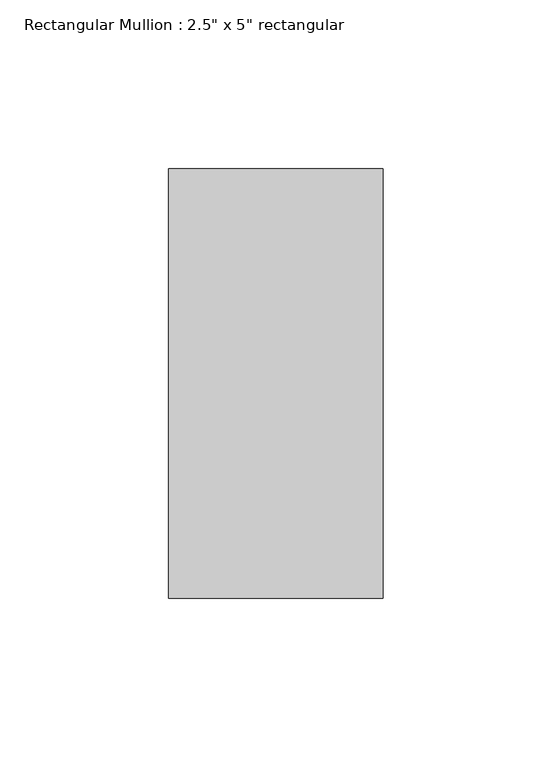
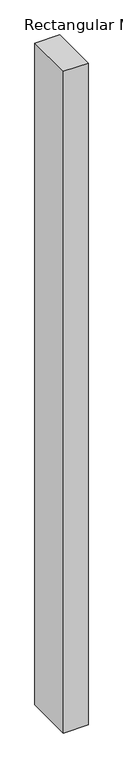
"""IFC4 building model written with IfcOpenShell, lengths in millimetres: member geometry."""

from ifc_helpers import new_model, si_unit, frame, origin, place, context, project, spatial, polyline, outline, extrude, source, transform, mapped, element, save


def member_5095b95d(model_context):
    return source(origin(), model_context, "Body", "SweptSolid", [
        extrude(outline(polyline([(31.75, 63.5), (31.75, -63.5), (-31.75, -63.5), (-31.75, 63.5), (31.75, 63.5)])), frame((0.0, 0.0, -1801.1599467), z_axis=(0.0, 0.0, 1.0), x_axis=(1.0, 0.0, 0.0)), (0.0, 0.0, 1.0), 1801.1599467),
    ])


if __name__ == "__main__":
    model = new_model("IFC4")
    model_context = context("Model", 3, world=origin())
    ifc_project = project(units=[si_unit("LENGTHUNIT", "METRE", prefix="MILLI")], contexts=[model_context])
    site = spatial("IfcSite", under=ifc_project)
    building = spatial("IfcBuilding", under=site)
    placement = place(None, origin())
    member_shape = member_5095b95d(model_context)
    element("IfcMember", 1, ObjectType="Rectangular Mullion : 2.5\" x 5\" rectangular", at=placement, inside=building, context=model_context, shape_type="MappedRepresentation", body=[
        mapped(member_shape, transform((0.0, 0.0, 0.0), x_axis=(1.0, 0.0, 0.0), y_axis=(0.0, 1.0, 0.0), z_axis=(0.0, 0.0, 1.0))),
    ])
    save(model, "model.ifc")

# Revit data of these elements
# Type "Rectangular Mullion : 2.5\" x 5\" rectangular"
#   built-in parameter 1007304 = 0.416667 (stored number, unit not read)
#   built-in parameter 1007301 = 0.104167 (stored number, unit not read)
#   built-in parameter 1007300 = 0.104167 (stored number, unit not read)
# Element 1 (IfcMember, "Rectangular Mullion : 2.5\" x 5\" rectangular")
#   Materials on its faces: "Aluminum"
# Materials
#   "Aluminum": class "Metal", colour RGB 247 247 247, transparency 0, Description = "Aluminum 6061", Cost = 0
